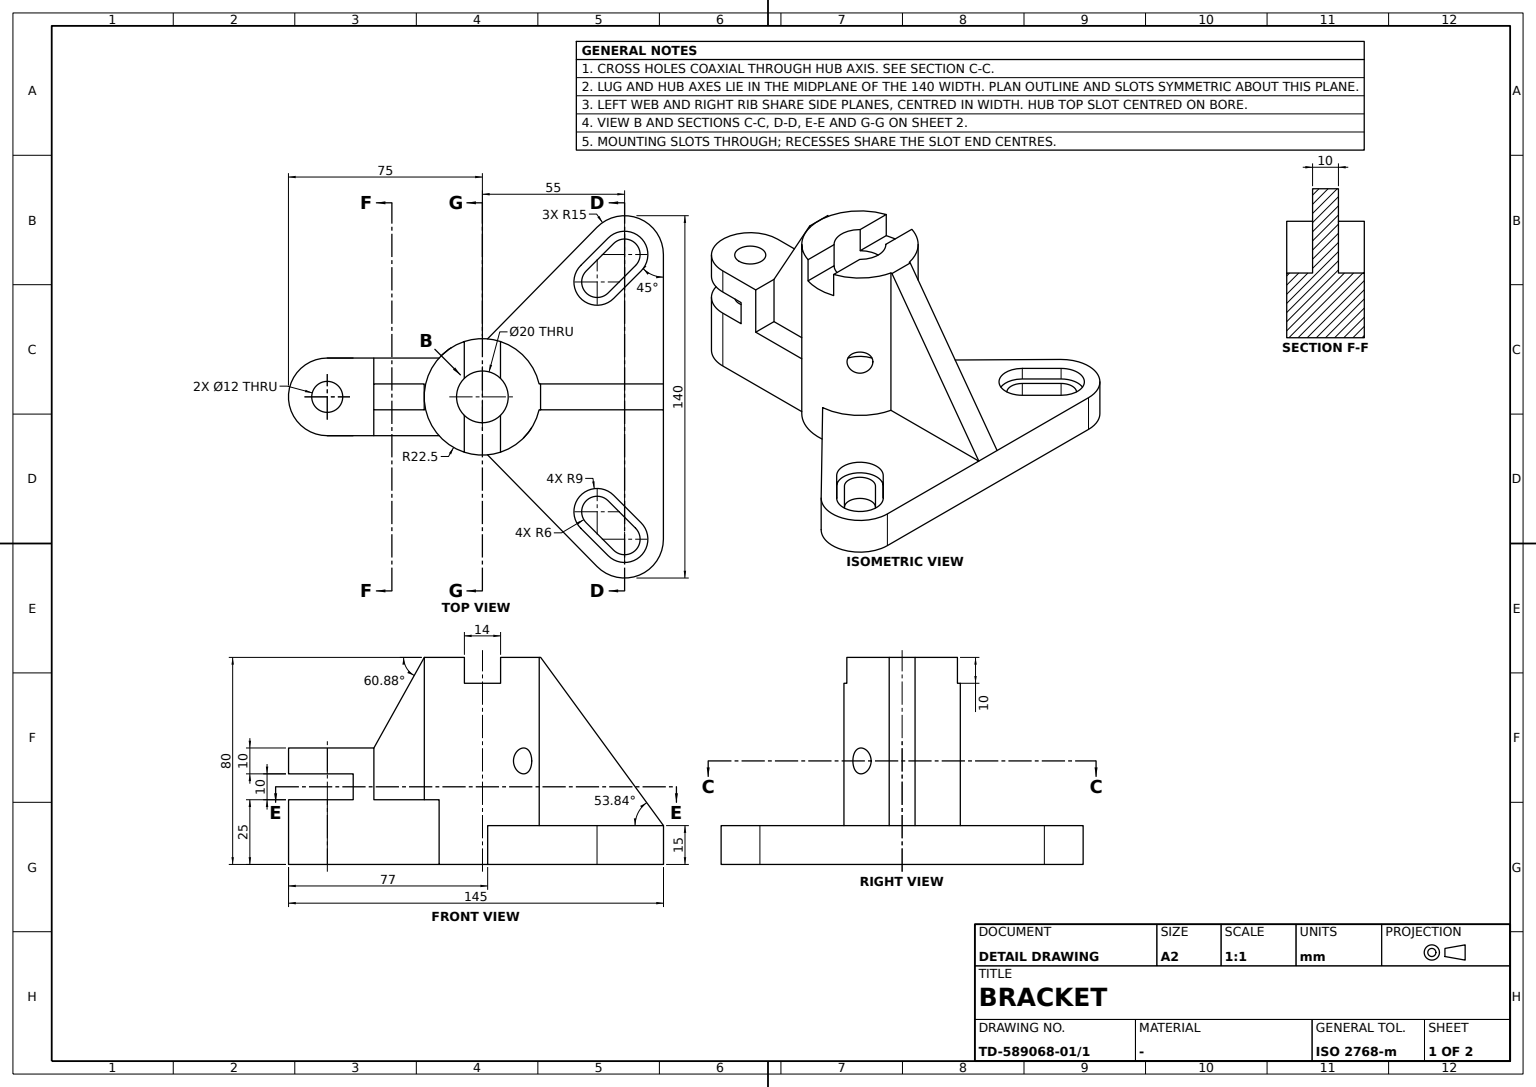
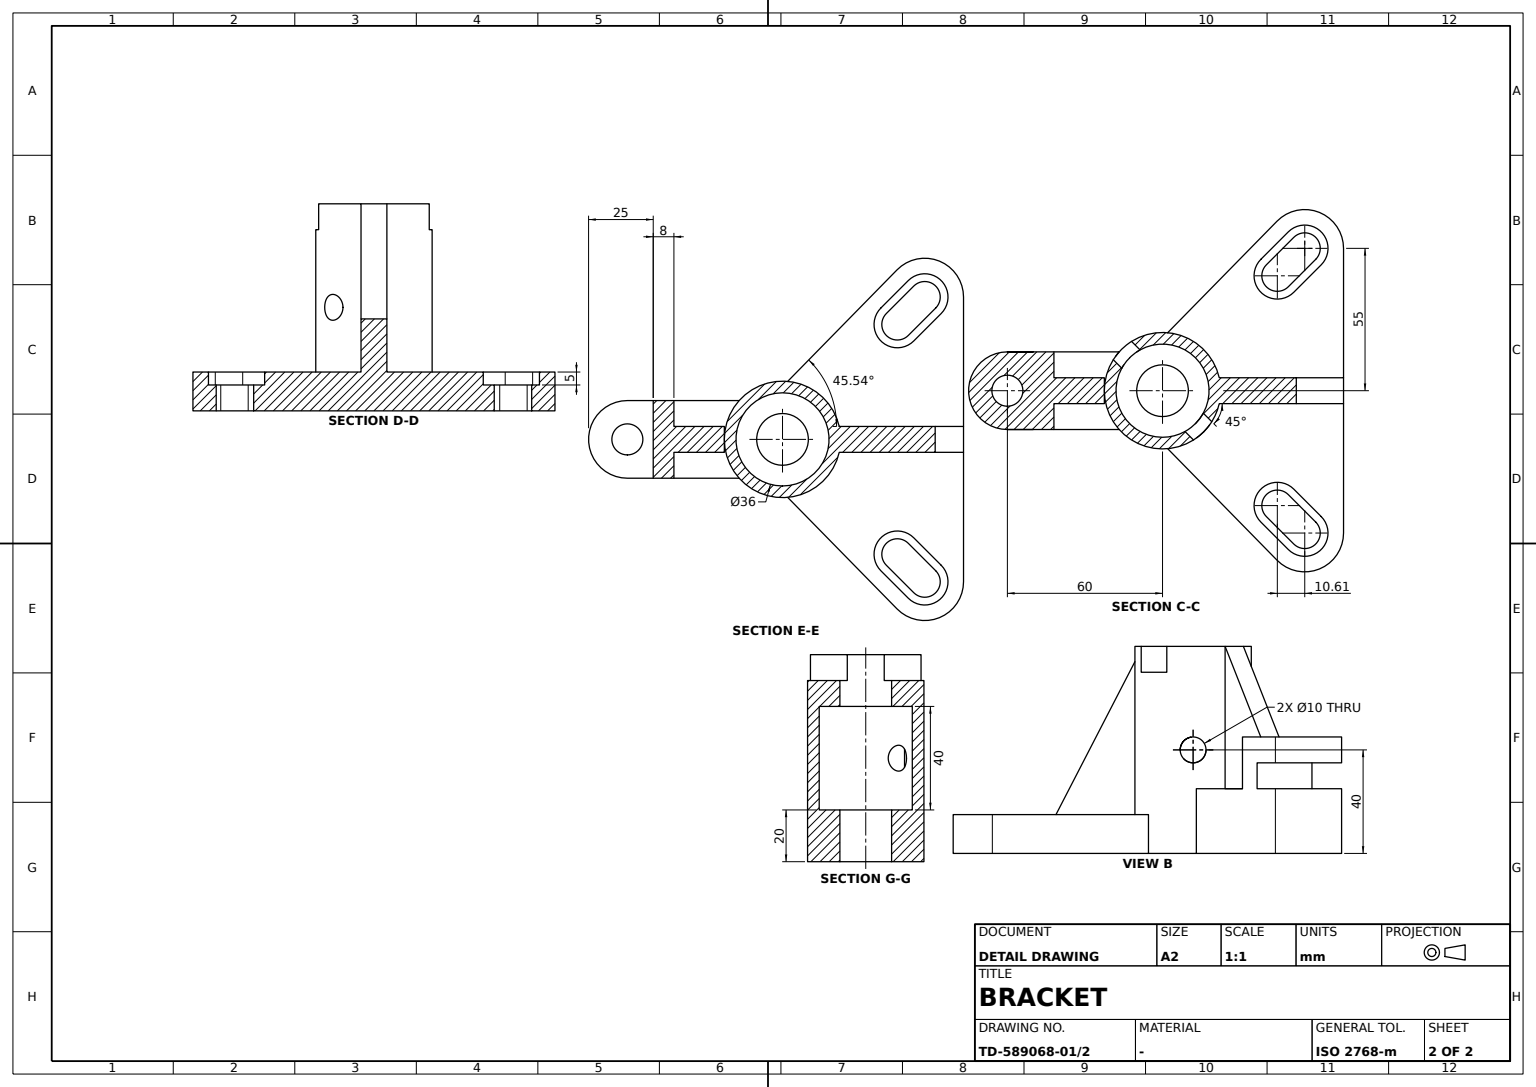
CATIA V5 part; units mm, degrees
sketch "Sketch1" plane through (0, 0, 0) normal (0, 0, 1) x (1, 0, 0)
  circle A0 centre (0, 0) radius 22.5
  circle A1 centre (0, 0) radius 10
  dimension "radius A1" = 10
  dimension "radius A0" = 22.5
extrude "Pad1" add sketch "Sketch1" along normal blind 80
sketch "Sketch2" plane through (0, 0, 0) normal (1, 0, 0) x (0, 1, 0)
  point P0 (0, 60)
  line L0 (0, 60) -> (18, 60)
  line L1 (18, 60) -> (18, 20)
  line L2 (18, 20) -> (0, 20)
  line L3 (0, 20) -> (0, 60)
  dimension "length L1" = 40
  dimension "distance L2 x axis" = 20
  dimension "length L0" = 18
  constraint coincidence P0 y-axis
  constraint horizontal L0 x-axis
  constraint horizontal L2 x-axis
  constraint vertical L1 y-axis
  constraint vertical L3 y-axis
revolve "Groove1" cut sketch "Sketch2" angle 360 about axis through (0, 0, 0) along (0, 0, 1)
sketch "Sketch3" plane through (0, 0, 0) normal (1, 0, 0) x (0, 1, 0)
  line L0 (-7, 81.1834) -> (7, 81.1834)
  line L1 (7, 81.1834) -> (7, 70)
  line L2 (7, 70) -> (-7, 70)
  line L3 (-7, 70) -> (-7, 81.1834)
  line L4 (-22.5, 80) -> (22.5, 80) construction
  dimension "length L0" = 14
  dimension "distance L2 L4" = 10
  constraint horizontal L0 x-axis
  constraint horizontal L2 x-axis
  constraint vertical L1 y-axis
  constraint vertical L3 y-axis
  constraint symmetry L3 L1 y-axis
extrude "Pocket1" cut sketch "Sketch3" against normal through all and the other way blind 80
ref_plane "Plane1" through (0, 0, 0) normal (0.7071, 0.7071, 0) x (-0.7071, 0.7071, 0)
sketch "Sketch4" plane through (0, 0, 0) normal (0.7071, 0.7071, 0) x (-0.7071, 0.7071, 0)
  circle A0 centre (0, 40) radius 5
  point P0 (0, 40)
  dimension "radius A0" = 5
  dimension "distance P0 x axis" = 40
  constraint coincidence P0 y-axis
extrude "Pocket2" cut sketch "Sketch4" along normal mid plane 49
sketch "Sketch5" plane through (0, 0, 0) normal (0, 0, 1) x (1, 0, 0)
  line L0 (55, 81.5988) -> (55, -81.5988) construction
  point P0 (55, 81.5988)
  point P1 (55, -81.5988)
  point P2 (69.8492, 57.1213)
  point P3 (2, -22.4109)
  point P4 (2, -22.4109)
  point P5 (-81.5988, 55)
  point P6 (-57.1213, 69.8492)
  point P7 (22.4109, 2)
  line L1 (-55, 70) -> (55, 70)
  line L2 (-22.4109, 2) -> (-9.798, 2)
  arc A0 (9.798, 2) -> (-9.798, 2) centre (0, 0) ccw
  line L3 (9.798, 2) -> (22.4109, 2)
  line L4 (-22.4109, 2) -> (-65.5066, 44.2943)
  arc A1 (-55, 70) -> (-65.5066, 44.2943) centre (-55, 55) ccw
  line L5 (22.4109, 2) -> (65.5066, 44.2943)
  arc A2 (55, 70) -> (65.5066, 44.2943) centre (55, 55) cw
  dimension "distance L0 y axis" = 55
  constraint vertical L0 y-axis
  constraint symmetry P0 P1 x-axis
  constraint coincidence P3 P4
extrude "Pad2" add sketch "Sketch5" along normal blind 15
sketch "Sketch6" plane through (0, 0, 0) normal (1, 0, 0) x (0, 1, 0)
  point P0 (22.501, 80)
  line L0 (22.501, 80) -> (22.501, 15)
  line L1 (22.501, 15) -> (70, 15)
  point P1 (70, 15)
  line L2 (70, 15) -> (22.501, 80)
  line L3 (-22.5, 80) -> (22.5, 80) construction
  line L4 (2, 15) -> (44.2943, 15) construction
  line L5 (70, 0) -> (70, 15) construction
  dimension "distance y axis L0" = 22.501
  constraint vertical L0 y-axis
  constraint horizontal L1 x-axis
  constraint coincidence P0 L3
  constraint coincidence L4 L1
  constraint coincidence P1 L5
extrude "Pad3" add sketch "Sketch6" along normal mid plane 10
sketch "Sketch7" plane through (0, 0, 80) normal (0, 0, 1) x (1, 0, 0)
  line L0 (-5, 22.501) -> (5, 22.501)
  arc A0 (21.3834, 7) -> (-21.3834, 7) centre (0, 0) ccw construction
  arc A1 (5, 21.9374) -> (-5, 21.9374) centre (0, 0) ccw
  line L1 (-5, 22.501) -> (-5, 21.9374)
  point P0 (-5, 21.9374)
  line L2 (5, 22.501) -> (5, 21.9374)
  point P1 (5, 21.9374)
  constraint coincidence P0 A0
  constraint coincidence P1 A0
  constraint vertical L1 y-axis
  constraint vertical L2 y-axis
extrude "Pad4" add sketch "Sketch7" against normal up to surface (65 mm away)
sketch "Sketch8" plane through (0, 0, 0) normal (0, 0, 1) x (1, 0, 0)
  line L0 (0, 0) -> (0, -60) construction
  arc A0 (-15, -60) -> (15, -60) centre (0, -60) ccw
  arc A1 (-21.3834, -7) -> (21.3834, -7) centre (0, 0) ccw construction
  arc A2 (-15, -16.7705) -> (15, -16.7705) centre (0, 0) ccw
  line L1 (-15, -60) -> (-15, -16.7705)
  point P0 (-15, -16.7705)
  line L2 (15, -60) -> (15, -16.7705)
  point P1 (15, -16.7705)
  point P2 (15, -60)
  point P3 (15, -60)
  dimension "length L0" = 60
  dimension "radius A0" = 15
  constraint vertical L0 y-axis
  constraint vertical L2 y-axis
  constraint vertical L1 y-axis
  constraint coincidence P0 A1
  constraint coincidence P1 A1
  constraint coincidence A0 P2
  constraint coincidence L2 P3
  constraint coincidence P2 P3
  constraint tangency L1 A0
  constraint tangency L2 A0
extrude "Pad5" add sketch "Sketch8" along normal blind 25
sketch "Sketch9" plane through (0, 0, 25) normal (0, 0, 1) x (1, 0, 0)
  arc A0 (-15, -60) -> (15, -60) centre (0, -60) ccw
  point P0 (0, -60)
  arc A1 (-15, -60) -> (15, -60) centre (0, -60) ccw construction
  arc A2 (-15, -60) -> (15, -60) centre (0, -60) ccw construction
  line L0 (-24.2907, -42) -> (28.1051, -42) construction
  line L1 (-15, -42) -> (-15, -60)
  line L2 (15, -42) -> (15, -60)
  point P1 (15, -42)
  line L3 (-15, -42) -> (15, -42)
  point P2 (-15, -42)
  point P3 (-15, -42)
  point P4 (15, -60)
  point P5 (15, -60)
  dimension "distance L0 P0" = 18
  constraint coincidence P0 y-axis
  constraint coincidence A0 A2
  constraint coincidence P1 L0
  constraint coincidence P2 L1
  constraint coincidence P2 L0
  constraint coincidence L0 P3
  constraint coincidence A0 P4
  constraint coincidence L2 P5
  constraint coincidence P2 P3
  constraint coincidence P4 P5
  constraint concentricity A0 A1
  constraint horizontal L0 x-axis
  constraint horizontal L3 x-axis
  constraint vertical L1 y-axis
  constraint vertical L2 y-axis
  constraint tangency L2 A0
  constraint tangency L1 A0
extrude "Pad6" add sketch "Sketch9" along normal blind 20
sketch "Sketch10" plane through (0, 0, 0) normal (1, 0, 0) x (0, 1, 0)
  point P0 (-42, 45)
  line L0 (-42, 45) -> (-42, 25)
  line L1 (-42, 25) -> (-22.5, 25)
  line L2 (-22.5, 25) -> (-22.5, 80)
  point P1 (-22.5, 80)
  line L3 (-22.5, 80) -> (-42, 45)
  line L4 (-22.5, 80) -> (22.5, 80) construction
  point P2 (-42, 45)
  line L5 (-60, 25) -> (-16.7705, 25) construction
  dimension "D1" = 22.5
  constraint vertical L0 y-axis
  constraint vertical L2 y-axis
  constraint horizontal L1 x-axis
  constraint coincidence P1 L4
  constraint coincidence P2 P0
  constraint coincidence L1 L5
extrude "Pad7" add sketch "Sketch10" along normal mid plane 10
sketch "Sketch11" plane through (0, 0, 45) normal (0, 0, 1) x (1, 0, 0)
  circle A0 centre (0, -60) radius 6
  point P0 (0, -60)
  point P1 (0, -66)
  arc A1 (-15, -60) -> (15, -60) centre (0, -60) ccw construction
  dimension "radius A0" = 6
  constraint coincidence P0 y-axis
  constraint coincidence A0 P1
  constraint coincidence P1 y-axis
  constraint concentricity A0 A1
extrude "Pocket3" cut sketch "Sketch11" against normal through all
sketch "Sketch12" plane through (0, 0, 0) normal (1, 0, 0) x (0, 1, 0)
  line L0 (-76.3987, 35) -> (-50, 35)
  line L1 (-50, 35) -> (-50, 25)
  line L2 (-50, 25) -> (-76.3987, 25)
  line L3 (-76.3987, 25) -> (-76.3987, 35)
  line L4 (-75, 45) -> (-60, 45) construction
  dimension "D1" = 10
  dimension "distance L0 L4" = 10
  dimension "length L3" = 10
  constraint horizontal L0 x-axis
  constraint horizontal L2 x-axis
  constraint vertical L1 y-axis
  constraint vertical L3 y-axis
extrude "Pocket4" cut sketch "Sketch12" along normal mid plane 44
sketch "Sketch13" plane through (0, 0, 15) normal (0, 0, 1) x (1, 0, 0)
  line L0 (-55, 55) -> (-44.3934, 44.3934) construction
  line L1 (-50.7574, 59.2426) -> (-40.1508, 48.636)
  line L2 (-48.636, 40.1508) -> (-59.2426, 50.7574)
  arc A0 (-40.1508, 48.636) -> (-48.636, 40.1508) centre (-44.3934, 44.3934) cw
  arc A1 (-59.2426, 50.7574) -> (-50.7574, 59.2426) centre (-55, 55) cw
  point P0 (-50.7574, 59.2426)
  point P1 (-40.1508, 48.636)
  point P2 (-48.636, 40.1508)
  point P3 (-59.2426, 50.7574)
  arc A2 (-55, 70) -> (-65.5066, 44.2943) centre (-55, 55) ccw construction
  line L3 (-55, 55) -> (-44.3934, 44.3934) construction
  line L4 (-48.636, 61.364) -> (-38.0294, 50.7574)
  line L5 (-50.7574, 38.0294) -> (-61.364, 48.636)
  arc A3 (-38.0294, 50.7574) -> (-50.7574, 38.0294) centre (-44.3934, 44.3934) cw
  arc A4 (-61.364, 48.636) -> (-48.636, 61.364) centre (-55, 55) cw
  point P4 (-48.636, 61.364)
  point P5 (-38.0294, 50.7574)
  point P6 (-50.7574, 38.0294)
  point P7 (-61.364, 48.636)
  line L6 (55, 55) -> (44.3934, 44.3934) construction
  point P8 (50.7574, 59.2426)
  point P9 (40.1508, 48.636)
  point P10 (48.636, 40.1508)
  point P11 (59.2426, 50.7574)
  line L7 (55, 55) -> (44.3934, 44.3934) construction
  point P12 (48.636, 61.364)
  point P13 (38.0294, 50.7574)
  point P14 (50.7574, 38.0294)
  point P15 (61.364, 48.636)
  line L8 (50.7574, 59.2426) -> (40.1508, 48.636)
  line L9 (48.636, 40.1508) -> (59.2426, 50.7574)
  arc A5 (40.1508, 48.636) -> (48.636, 40.1508) centre (44.3934, 44.3934) ccw
  arc A6 (59.2426, 50.7574) -> (50.7574, 59.2426) centre (55, 55) ccw
  line L10 (48.636, 61.364) -> (38.0294, 50.7574)
  line L11 (50.7574, 38.0294) -> (61.364, 48.636)
  arc A7 (38.0294, 50.7574) -> (50.7574, 38.0294) centre (44.3934, 44.3934) ccw
  arc A8 (61.364, 48.636) -> (48.636, 61.364) centre (55, 55) ccw
  dimension "distance L0 L1" = 6
  dimension "length L0" = 15
  dimension "distance L3 L4" = 9
  dimension "angle L3 y axis" = 45
  constraint tangency A0 L1
  constraint tangency A1 L1
  constraint tangency A0 L2
  constraint tangency A1 L2
  constraint tangency A3 L4
  constraint tangency A4 L4
  constraint tangency A3 L5
  constraint tangency A4 L5
  constraint concentricity A1 A2
  constraint parallelism L3 L0
  constraint symmetry L0 L6 y-axis
  constraint symmetry P0 P8 y-axis
  constraint symmetry P1 P9 y-axis
  constraint symmetry P2 P10 y-axis
  constraint symmetry P3 P11 y-axis
  constraint symmetry L3 L7 y-axis
  constraint symmetry P4 P12 y-axis
  constraint symmetry P5 P13 y-axis
  constraint symmetry P6 P14 y-axis
  constraint symmetry P7 P15 y-axis
  constraint symmetry L1 L8 y-axis
  constraint symmetry L2 L9 y-axis
  constraint symmetry A0 A5 y-axis
  constraint symmetry A1 A6 y-axis
  constraint symmetry L4 L10 y-axis
  constraint symmetry L5 L11 y-axis
  constraint symmetry A3 A7 y-axis
  constraint symmetry A4 A8 y-axis
extrude "MultiPocket1 domain 1" cut sketch "Sketch13" against normal blind 5 contours L10 A7 L11 A8
extrude "MultiPocket1 domain 2" cut sketch "Sketch13" against normal blind 20 contours L8 A5 L9 A6
extrude "MultiPocket1 domain 3" cut sketch "Sketch13" against normal blind 5 contours L4 A3 L5 A4
extrude "MultiPocket1 domain 4" cut sketch "Sketch13" against normal blind 20 contours L1 A0 L2 A1
properties part number "23"
